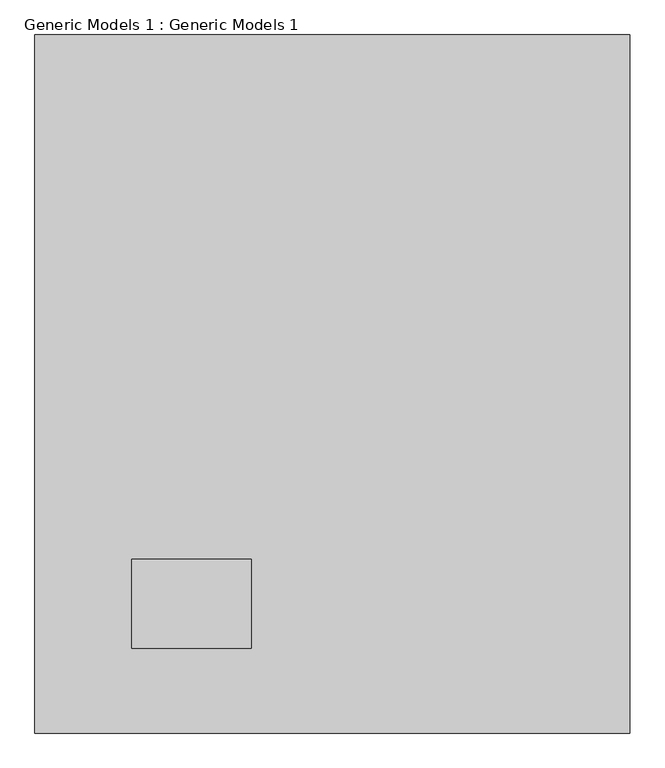
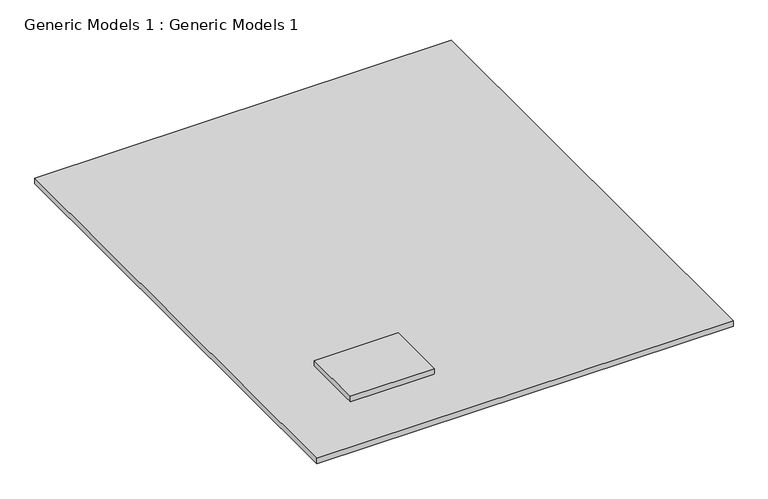
"""IFC4 building model written with IfcOpenShell, lengths in millimetres: proxy geometry, Generic Models 1 : Generic Models 1."""

from ifc_helpers import new_model, si_unit, frame, origin, origin_with_axes, place, context, project, spatial, polyline, outline, extrude, source, transform, mapped, element, save


def generic_models_1_generic_models_1_3e26791c(model_context):
    return source(origin(), model_context, "Body", "SweptSolid", [
        extrude(outline(polyline([(-759.6702714, 10702.4410241), (-759.6702714, -14673.8383903), (-22379.5962313, -14673.8383903), (-22379.5962313, 10702.4410241), (-759.6702714, 10702.4410241)])), frame((0.0, 0.0, -304.8), z_axis=(0.0, 0.0, 1.0), x_axis=(1.0, 0.0, 0.0)), (0.0, 0.0, 1.0), 304.8),
        extrude(outline(polyline([(-14513.7702714, -8349.2383903), (-14513.7702714, -11587.7383903), (-18857.1702714, -11587.7383903), (-18857.1702714, -8349.2383903), (-14513.7702714, -8349.2383903)])), origin_with_axes(), (0.0, 0.0, 1.0), 304.8),
    ])


if __name__ == "__main__":
    model = new_model("IFC4")
    model_context = context("Model", 3, world=origin())
    ifc_project = project(units=[si_unit("LENGTHUNIT", "METRE", prefix="MILLI")], contexts=[model_context])
    site = spatial("IfcSite", under=ifc_project)
    building = spatial("IfcBuilding", under=site)
    placement = place(None, origin())
    generic_models_1_generic_models_1_shape = generic_models_1_generic_models_1_3e26791c(model_context)
    element("IfcBuildingElementProxy", 1, Name="Generic Models 1 : Generic Models 1", ObjectType="Generic Models 1 : Generic Models 1", at=placement, inside=building, context=model_context, shape_type="MappedRepresentation", body=[
        mapped(generic_models_1_generic_models_1_shape, transform((0.0, 0.0, 0.0), x_axis=(1.0, 0.0, 0.0), y_axis=(0.0, 1.0, 0.0), z_axis=(0.0, 0.0, 1.0))),
    ])
    save(model, "model.ifc")
